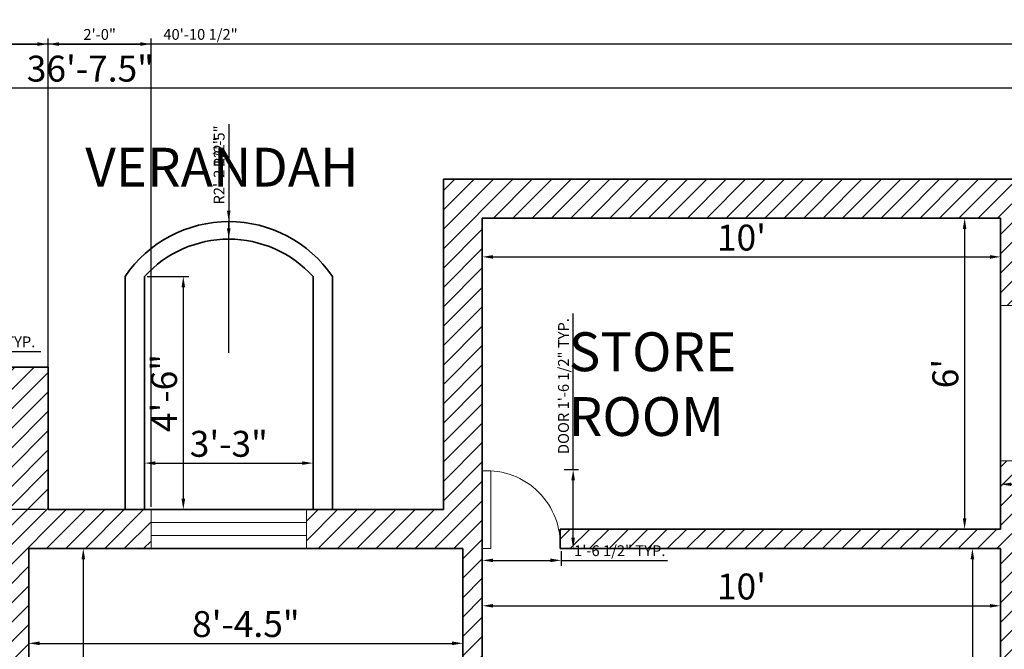
# Model space of a CAD drawing. Units: inches. Extents: x 4740 to 5323, y 7115 to 7713.
# Tile 5 of 6: x 4980 to 5208, y 7567 to 7713. Entities that reach past the tile are written whole.
import ezdxf

# ---------------------------------------------------------------- set-up
doc = ezdxf.new("R2010")
doc.units = ezdxf.units.IN
for name, color, linetype, lineweight in [('A-ANNO-DIMS', 2, 'Continuous', 18), ('A-AREA-IDEN', 7, 'Continuous', 25), ('A-DOOR', 4, 'Continuous', 18), ('A-GLAZ', 242, 'Continuous', 18), ('A-WALL', 7, 'Continuous', 35)]:
    doc.layers.add(name, color=color, linetype=linetype, lineweight=lineweight)
doc.layers.add('A-WALL-PATT', color=152, linetype='Continuous', lineweight=13, true_color=0x2776bb)
doc.styles.get("Standard").update_dxf_attribs({"font": 'arial.ttf'})
doc.dimstyles.new('ISO-25', dxfattribs={"dimtxt": 2.5, "dimasz": 2.5, "dimexe": 1.25, "dimexo": 0.625, "dimtad": 1, "dimlunit": 3, "dimtxsty": 'Standard', "dimcen": 2.5, "dimadec": 0, "dimazin": 0, "dimtfac": 1, "dimtmove": 0, "dimatfit": 3, "dimfxl": 1, "dimarcsym": 0})

# ---------------------------------------------------------------- blocks, each defined once
blk = doc.blocks.new('*D17')
at = {"layer": 'A-ANNO-DIMS', "color": 0, "lineweight": -2, "transparency": 16777216}
for p, q in [((5009.38, 7653.36), (5018.98, 7653.36)), ((5017.73, 7650.86), (5017.73, 7601.86)), ((5009.38, 7599.36), (5018.98, 7599.36))]:
    blk.add_line(p, q, dxfattribs=at)
at = {"layer": 'A-ANNO-DIMS', "color": 0, "transparency": 16777216}
for points in [[(5017.32, 7650.86), (5018.15, 7650.86), (5017.73, 7653.36)], [(5017.32, 7601.86), (5018.15, 7601.86), (5017.73, 7599.36)]]:
    blk.add_solid(points, dxfattribs=at)
at = {"layer": 'Defpoints', "color": 0, "transparency": 16777216}
for p in [(5008.76, 7653.36), (5008.76, 7599.36), (5017.73, 7599.36)]:
    blk.add_point(p, dxfattribs=at)
at = {"layer": 'A-ANNO-DIMS', "color": 0, "transparency": 16777216, "insert": (5014.05, 7626.36), "char_height": 6, "attachment_point": 5, "rotation": 90}
blk.add_mtext('4\'-6"', dxfattribs=at)
blk = doc.blocks.new('*D18')
at = {"layer": 'A-ANNO-DIMS', "color": 0, "lineweight": -2, "transparency": 16777216}
for p, q in [((5008.76, 7599.98), (5008.76, 7611.38)), ((5047.76, 7599.98), (5047.76, 7611.38)), ((5011.26, 7610.13), (5045.26, 7610.13))]:
    blk.add_line(p, q, dxfattribs=at)
at = {"layer": 'A-ANNO-DIMS', "color": 0, "transparency": 16777216}
for points in [[(5011.26, 7610.54), (5011.26, 7609.71), (5008.76, 7610.13)], [(5045.26, 7610.54), (5045.26, 7609.71), (5047.76, 7610.13)]]:
    blk.add_solid(points, dxfattribs=at)
at = {"layer": 'Defpoints', "color": 0, "transparency": 16777216}
for p in [(5047.76, 7610.13), (5008.76, 7599.36), (5047.76, 7599.36)]:
    blk.add_point(p, dxfattribs=at)
at = {"layer": 'A-ANNO-DIMS', "color": 0, "transparency": 16777216, "insert": (5028.26, 7613.82), "char_height": 6, "attachment_point": 5}
blk.add_mtext('3\'-3"', dxfattribs=at)
blk = doc.blocks.new('*D19')
at = {"layer": 'A-ANNO-DIMS', "color": 0, "lineweight": -2, "transparency": 16777216}
for p, q in [((5086.96, 7666.23), (5086.96, 7656.63)), ((5206.96, 7666.23), (5206.96, 7656.63)), ((5089.46, 7657.88), (5204.46, 7657.88))]:
    blk.add_line(p, q, dxfattribs=at)
at = {"layer": 'A-ANNO-DIMS', "color": 0, "transparency": 16777216}
for points in [[(5089.46, 7658.29), (5089.46, 7657.46), (5086.96, 7657.88)], [(5204.46, 7658.29), (5204.46, 7657.46), (5206.96, 7657.88)]]:
    blk.add_solid(points, dxfattribs=at)
at = {"layer": 'Defpoints', "color": 0, "transparency": 16777216}
for p in [(5086.96, 7666.86), (5206.96, 7666.86), (5206.96, 7657.88)]:
    blk.add_point(p, dxfattribs=at)
at = {"layer": 'A-ANNO-DIMS', "color": 0, "transparency": 16777216, "insert": (5146.96, 7661.57), "char_height": 6, "attachment_point": 5}
blk.add_mtext("10'", dxfattribs=at)
blk = doc.blocks.new('*D20')
at = {"layer": 'A-ANNO-DIMS', "color": 0, "lineweight": -2, "transparency": 16777216}
for p, q in [((5206.33, 7666.86), (5197.37, 7666.86)), ((5198.62, 7664.36), (5198.62, 7597.36)), ((5206.33, 7594.86), (5197.37, 7594.86))]:
    blk.add_line(p, q, dxfattribs=at)
at = {"layer": 'A-ANNO-DIMS', "color": 0, "transparency": 16777216}
for points in [[(5198.2, 7664.36), (5199.03, 7664.36), (5198.62, 7666.86)], [(5198.2, 7597.36), (5199.03, 7597.36), (5198.62, 7594.86)]]:
    blk.add_solid(points, dxfattribs=at)
at = {"layer": 'Defpoints', "color": 0, "transparency": 16777216}
for p in [(5206.96, 7666.86), (5198.62, 7594.86), (5206.96, 7594.86)]:
    blk.add_point(p, dxfattribs=at)
at = {"layer": 'A-ANNO-DIMS', "color": 0, "transparency": 16777216, "insert": (5194.93, 7630.86), "char_height": 6, "attachment_point": 5, "rotation": 90}
blk.add_mtext("6'", dxfattribs=at)
blk = doc.blocks.new('*D21')
at = {"layer": 'A-ANNO-DIMS', "color": 0, "lineweight": -2, "transparency": 16777216}
for p, q in [((5086.96, 7589.73), (5086.96, 7575.84)), ((5206.96, 7589.73), (5206.96, 7575.84)), ((5089.46, 7577.09), (5204.46, 7577.09))]:
    blk.add_line(p, q, dxfattribs=at)
at = {"layer": 'A-ANNO-DIMS', "color": 0, "transparency": 16777216}
for points in [[(5089.46, 7577.51), (5089.46, 7576.68), (5086.96, 7577.09)], [(5204.46, 7577.51), (5204.46, 7576.68), (5206.96, 7577.09)]]:
    blk.add_solid(points, dxfattribs=at)
at = {"layer": 'Defpoints', "color": 0, "transparency": 16777216}
for p in [(5086.96, 7590.36), (5206.96, 7590.36), (5206.96, 7577.09)]:
    blk.add_point(p, dxfattribs=at)
at = {"layer": 'A-ANNO-DIMS', "color": 0, "transparency": 16777216, "insert": (5146.96, 7580.78), "char_height": 6, "attachment_point": 5}
blk.add_mtext("10'", dxfattribs=at)
blk = doc.blocks.new('*D22')
at = {"layer": 'A-ANNO-DIMS', "color": 0, "lineweight": -2, "transparency": 16777216}
for p, q in [((5206.33, 7590.36), (5199.17, 7590.36)), ((5200.42, 7587.86), (5200.42, 7429.36)), ((5206.33, 7426.86), (5199.17, 7426.86))]:
    blk.add_line(p, q, dxfattribs=at)
at = {"layer": 'A-ANNO-DIMS', "color": 0, "transparency": 16777216}
for points in [[(5200, 7587.86), (5200.84, 7587.86), (5200.42, 7590.36)], [(5200, 7429.36), (5200.84, 7429.36), (5200.42, 7426.86)]]:
    blk.add_solid(points, dxfattribs=at)
at = {"layer": 'Defpoints', "color": 0, "transparency": 16777216}
for p in [(5206.96, 7590.36), (5200.42, 7426.86), (5206.96, 7426.86)]:
    blk.add_point(p, dxfattribs=at)
at = {"layer": 'A-ANNO-DIMS', "color": 0, "transparency": 16777216, "insert": (5196.73, 7508.61), "char_height": 6, "attachment_point": 5, "rotation": 90}
blk.add_mtext('13\'-7.5"', dxfattribs=at)
blk = doc.blocks.new('*D32')
at = {"layer": 'A-ANNO-DIMS', "color": 0, "lineweight": -2, "transparency": 16777216}
for p, q in [((4982.58, 7590.36), (4995.83, 7590.36)), ((4994.58, 7587.86), (4994.58, 7429.36)), ((4982.58, 7426.86), (4995.83, 7426.86))]:
    blk.add_line(p, q, dxfattribs=at)
at = {"layer": 'A-ANNO-DIMS', "color": 0, "transparency": 16777216}
for points in [[(4994.17, 7587.86), (4995, 7587.86), (4994.58, 7590.36)], [(4994.17, 7429.36), (4995, 7429.36), (4994.58, 7426.86)]]:
    blk.add_solid(points, dxfattribs=at)
at = {"layer": 'Defpoints', "color": 0, "transparency": 16777216}
for p in [(4981.96, 7590.36), (4981.96, 7426.86), (4994.58, 7426.86)]:
    blk.add_point(p, dxfattribs=at)
at = {"layer": 'A-ANNO-DIMS', "color": 0, "transparency": 16777216, "insert": (4990.89, 7508.61), "char_height": 6, "attachment_point": 5, "rotation": 90}
blk.add_mtext('13\'-7.5"', dxfattribs=at)
blk = doc.blocks.new('*D33')
at = {"layer": 'A-ANNO-DIMS', "color": 0, "lineweight": -2, "transparency": 16777216}
for p, q in [((4981.96, 7589.73), (4981.96, 7567.15)), ((5082.46, 7589.73), (5082.46, 7567.15)), ((4984.46, 7568.4), (5079.96, 7568.4))]:
    blk.add_line(p, q, dxfattribs=at)
at = {"layer": 'A-ANNO-DIMS', "color": 0, "transparency": 16777216}
for points in [[(4984.46, 7568.82), (4984.46, 7567.98), (4981.96, 7568.4)], [(5079.96, 7568.82), (5079.96, 7567.98), (5082.46, 7568.4)]]:
    blk.add_solid(points, dxfattribs=at)
at = {"layer": 'Defpoints', "color": 0, "transparency": 16777216}
for p in [(4981.96, 7590.36), (5082.46, 7590.36), (5082.46, 7568.4)]:
    blk.add_point(p, dxfattribs=at)
at = {"layer": 'A-ANNO-DIMS', "color": 0, "transparency": 16777216, "insert": (5032.21, 7572.09), "char_height": 6, "attachment_point": 5}
blk.add_mtext('8\'-4.5"', dxfattribs=at)
blk = doc.blocks.new('*D35')
at = {"layer": 'A-ANNO-DIMS', "color": 0, "lineweight": -2, "transparency": 16777216}
for p, q in [((4776.46, 7632.98), (4776.46, 7698.25)), ((5215.96, 7629.25), (5215.96, 7698.25)), ((4778.96, 7697), (5213.46, 7697))]:
    blk.add_line(p, q, dxfattribs=at)
at = {"layer": 'A-ANNO-DIMS', "color": 0, "transparency": 16777216}
for points in [[(4778.96, 7697.42), (4778.96, 7696.58), (4776.46, 7697)], [(5213.46, 7697.42), (5213.46, 7696.58), (5215.96, 7697)]]:
    blk.add_solid(points, dxfattribs=at)
at = {"layer": 'Defpoints', "color": 0, "transparency": 16777216}
for p in [(5215.96, 7697), (4776.46, 7632.36), (5215.96, 7628.62)]:
    blk.add_point(p, dxfattribs=at)
at = {"layer": 'A-ANNO-DIMS', "color": 0, "transparency": 16777216, "insert": (4996.21, 7700.69), "char_height": 6, "attachment_point": 5}
blk.add_mtext('36\'-7.5"', dxfattribs=at)
blk = doc.blocks.new('*D36')
at = {"layer": 'A-ANNO-DIMS', "color": 0, "lineweight": -2, "transparency": 16777216}
for p, q in [((5078.58, 7675.86), (5323.05, 7675.86)), ((5321.8, 7673.36), (5321.8, 7150.66)), ((5077.56, 7148.16), (5323.05, 7148.16))]:
    blk.add_line(p, q, dxfattribs=at)
at = {"layer": 'A-ANNO-DIMS', "color": 0, "transparency": 16777216}
for points in [[(5321.38, 7673.36), (5322.22, 7673.36), (5321.8, 7675.86)], [(5321.38, 7150.66), (5322.22, 7150.66), (5321.8, 7148.16)]]:
    blk.add_solid(points, dxfattribs=at)
at = {"layer": 'Defpoints', "color": 0, "transparency": 16777216}
for p in [(5077.96, 7675.86), (5076.93, 7148.16), (5321.8, 7148.16)]:
    blk.add_point(p, dxfattribs=at)
at = {"layer": 'A-ANNO-DIMS', "color": 0, "transparency": 16777216, "insert": (5318.11, 7412.01), "char_height": 6, "attachment_point": 5, "rotation": 90}
blk.add_mtext('43\'-11.7"', dxfattribs=at)
blk = doc.blocks.new('WIN-36IN')
for p, q in [((0, 36), (9, 36)), ((0, 36), (0, 0)), ((3, 36), (3, 0)), ((6, 36), (6, 0)), ((9, 0), (9, 36)), ((0, 0), (9, 0))]:
    blk.add_line(p, q)
blk = doc.blocks.new('DOOR-SWING-18IN')
for p, q in [((0, 0), (0, 18)), ((0, 18), (2, 18)), ((2, 18), (2, 0)), ((2, 0), (0, 0))]:
    blk.add_line(p, q)
blk.add_arc((1, 1), 17.03, 356.6335, 93.3665)
blk = doc.blocks.new('*D44')
at = {"layer": 'A-ANNO-DIMS', "color": 0, "lineweight": -2, "transparency": 16777216}
for p, q in [((4925.34, 7632.98), (4925.34, 7637.21)), ((4949.34, 7632.98), (4949.34, 7637.21)), ((4927.84, 7635.96), (4946.84, 7635.96)), ((4949.34, 7635.96), (4984.73, 7635.96))]:
    blk.add_line(p, q, dxfattribs=at)
at = {"layer": 'A-ANNO-DIMS', "color": 0, "transparency": 16777216}
for points in [[(4927.84, 7636.37), (4927.84, 7635.54), (4925.34, 7635.96)], [(4946.84, 7636.37), (4946.84, 7635.54), (4949.34, 7635.96)]]:
    blk.add_solid(points, dxfattribs=at)
at = {"layer": 'Defpoints', "color": 0, "transparency": 16777216}
for p in [(4949.34, 7635.96), (4925.34, 7632.36), (4949.34, 7632.36)]:
    blk.add_point(p, dxfattribs=at)
at = {"layer": 'A-ANNO-DIMS', "color": 0, "transparency": 16777216, "insert": (4968.29, 7637.88), "char_height": 2.5, "attachment_point": 5}
blk.add_mtext('WINDOW 2\'-0" TYP.', dxfattribs=at)
blk = doc.blocks.new('*D47')
at = {"layer": 'A-ANNO-DIMS', "color": 0, "lineweight": -2, "transparency": 16777216}
for p, q in [((5206.96, 7610), (5206.96, 7603.97)), ((5215.96, 7610), (5215.96, 7603.97)), ((5209.46, 7605.22), (5213.46, 7605.22)), ((5215.96, 7605.22), (5234.95, 7605.22))]:
    blk.add_line(p, q, dxfattribs=at)
at = {"layer": 'A-ANNO-DIMS', "color": 0, "transparency": 16777216}
for points in [[(5209.46, 7605.64), (5209.46, 7604.81), (5206.96, 7605.22)], [(5213.46, 7605.64), (5213.46, 7604.81), (5215.96, 7605.22)]]:
    blk.add_solid(points, dxfattribs=at)
at = {"layer": 'Defpoints', "color": 0, "transparency": 16777216}
for p in [(5206.96, 7610.62), (5215.96, 7610.62), (5215.96, 7605.22)]:
    blk.add_point(p, dxfattribs=at)
at = {"layer": 'A-ANNO-DIMS', "color": 0, "transparency": 16777216, "insert": (5226.7, 7607.13), "char_height": 2.5, "attachment_point": 5}
blk.add_mtext('0\'-9" TYP.', dxfattribs=at)
blk = doc.blocks.new('*D56')
at = {"layer": 'A-ANNO-DIMS', "color": 0, "lineweight": -2, "transparency": 16777216}
for p, q in [((5107.99, 7608.64), (5107.99, 7644.78)), ((5105.87, 7608.64), (5109.24, 7608.64)), ((5107.99, 7592.86), (5107.99, 7606.14)), ((5105.87, 7590.36), (5109.24, 7590.36))]:
    blk.add_line(p, q, dxfattribs=at)
at = {"layer": 'A-ANNO-DIMS', "color": 0, "transparency": 16777216}
for points in [[(5107.57, 7606.14), (5108.4, 7606.14), (5107.99, 7608.64)], [(5107.57, 7592.86), (5108.4, 7592.86), (5107.99, 7590.36)]]:
    blk.add_solid(points, dxfattribs=at)
at = {"layer": 'Defpoints', "color": 0, "transparency": 16777216}
for p in [(5105.24, 7608.64), (5107.99, 7608.64), (5105.24, 7590.36)]:
    blk.add_point(p, dxfattribs=at)
at = {"layer": 'A-ANNO-DIMS', "color": 0, "transparency": 16777216, "insert": (5106.07, 7627.96), "char_height": 2.5, "attachment_point": 5, "rotation": 90}
blk.add_mtext('DOOR 1\'-6 1/2" TYP.', dxfattribs=at)
blk = doc.blocks.new('*D57')
at = {"layer": 'A-ANNO-DIMS', "color": 0, "lineweight": -2, "transparency": 16777216}
for p, q in [((5086.96, 7589.73), (5086.96, 7586.36)), ((5105.24, 7589.73), (5105.24, 7586.36)), ((5089.46, 7587.61), (5102.74, 7587.61)), ((5105.24, 7587.61), (5129.82, 7587.61))]:
    blk.add_line(p, q, dxfattribs=at)
at = {"layer": 'A-ANNO-DIMS', "color": 0, "transparency": 16777216}
for points in [[(5089.46, 7588.03), (5089.46, 7587.2), (5086.96, 7587.61)], [(5102.74, 7588.03), (5102.74, 7587.2), (5105.24, 7587.61)]]:
    blk.add_solid(points, dxfattribs=at)
at = {"layer": 'Defpoints', "color": 0, "transparency": 16777216}
for p in [(5086.96, 7590.36), (5105.24, 7590.36), (5105.24, 7587.61)]:
    blk.add_point(p, dxfattribs=at)
at = {"layer": 'A-ANNO-DIMS', "color": 0, "transparency": 16777216, "insert": (5118.78, 7589.53), "char_height": 2.5, "attachment_point": 5}
blk.add_mtext('1\'-6 1/2" TYP.', dxfattribs=at)
blk = doc.blocks.new('*D74')
at = {"layer": 'A-ANNO-DIMS', "color": 0, "lineweight": -2, "transparency": 16777216}
for p, q in [((4949.34, 7632.98), (4949.34, 7708.41)), ((4951.84, 7707.16), (4983.96, 7707.16)), ((4986.46, 7632.98), (4986.46, 7708.41))]:
    blk.add_line(p, q, dxfattribs=at)
at = {"layer": 'A-ANNO-DIMS', "color": 0, "transparency": 16777216}
for points in [[(4951.84, 7707.57), (4951.84, 7706.74), (4949.34, 7707.16)], [(4983.96, 7707.57), (4983.96, 7706.74), (4986.46, 7707.16)]]:
    blk.add_solid(points, dxfattribs=at)
at = {"layer": 'Defpoints', "color": 0, "transparency": 16777216}
for p in [(4986.46, 7707.16), (4949.34, 7632.36), (4986.46, 7632.36)]:
    blk.add_point(p, dxfattribs=at)
at = {"layer": 'A-ANNO-DIMS', "color": 0, "transparency": 16777216, "insert": (4967.9, 7709.06), "char_height": 2.5, "attachment_point": 5}
blk.add_mtext('3\'-1"', dxfattribs=at)
blk = doc.blocks.new('*D80')
at = {"layer": 'A-ANNO-DIMS', "color": 0, "lineweight": -2, "transparency": 16777216}
for p, q in [((4986.46, 7599.98), (4986.46, 7708.41)), ((4988.96, 7707.16), (5007.76, 7707.16)), ((5010.26, 7599.98), (5010.26, 7708.41))]:
    blk.add_line(p, q, dxfattribs=at)
at = {"layer": 'A-ANNO-DIMS', "color": 0, "transparency": 16777216}
for points in [[(4988.96, 7707.57), (4988.96, 7706.74), (4986.46, 7707.16)], [(5007.76, 7707.57), (5007.76, 7706.74), (5010.26, 7707.16)]]:
    blk.add_solid(points, dxfattribs=at)
at = {"layer": 'Defpoints', "color": 0, "transparency": 16777216}
for p in [(5010.26, 7707.16), (4986.46, 7599.36), (5010.26, 7599.36)]:
    blk.add_point(p, dxfattribs=at)
at = {"layer": 'A-ANNO-DIMS', "color": 0, "transparency": 16777216, "insert": (4998.36, 7709.06), "char_height": 2.5, "attachment_point": 5}
blk.add_mtext('2\'-0"', dxfattribs=at)
blk = doc.blocks.new('*D81')
at = {"layer": 'A-ANNO-DIMS', "color": 0, "lineweight": -2, "transparency": 16777216}
for p, q in [((4776.46, 7632.98), (4776.46, 7708.41)), ((5264.46, 7707.16), (4778.96, 7707.16)), ((5266.96, 7422.98), (5266.96, 7708.41))]:
    blk.add_line(p, q, dxfattribs=at)
at = {"layer": 'A-ANNO-DIMS', "color": 0, "transparency": 16777216}
for points in [[(4778.96, 7707.57), (4778.96, 7706.74), (4776.46, 7707.16)], [(5264.46, 7707.57), (5264.46, 7706.74), (5266.96, 7707.16)]]:
    blk.add_solid(points, dxfattribs=at)
at = {"layer": 'Defpoints', "color": 0, "transparency": 16777216}
for p in [(4776.46, 7707.16), (4776.46, 7632.36), (5266.96, 7422.36)]:
    blk.add_point(p, dxfattribs=at)
at = {"layer": 'A-ANNO-DIMS', "color": 0, "transparency": 16777216, "insert": (5021.71, 7709.07), "char_height": 2.5, "attachment_point": 5}
blk.add_mtext('40\'-10 1/2"', dxfattribs=at)
blk = doc.blocks.new('*D82')
at = {"layer": 'A-ANNO-DIMS', "color": 0, "lineweight": -2, "transparency": 16777216}
for p, q in [((4985.83, 7632.36), (4743.91, 7632.36)), ((4745.16, 7629.86), (4745.16, 7601.86)), ((4985.83, 7599.36), (4743.91, 7599.36))]:
    blk.add_line(p, q, dxfattribs=at)
at = {"layer": 'A-ANNO-DIMS', "color": 0, "transparency": 16777216}
for points in [[(4744.74, 7629.86), (4745.58, 7629.86), (4745.16, 7632.36)], [(4744.74, 7601.86), (4745.58, 7601.86), (4745.16, 7599.36)]]:
    blk.add_solid(points, dxfattribs=at)
at = {"layer": 'Defpoints', "color": 0, "transparency": 16777216}
for p in [(4986.46, 7632.36), (4745.16, 7599.36), (4986.46, 7599.36)]:
    blk.add_point(p, dxfattribs=at)
at = {"layer": 'A-ANNO-DIMS', "color": 0, "transparency": 16777216, "insert": (4743.26, 7615.86), "char_height": 2.5, "attachment_point": 5, "rotation": 90}
blk.add_mtext('2\'-9"', dxfattribs=at)
blk = doc.blocks.new('*D86')
at = {"layer": 'A-ANNO-DIMS', "color": 0, "lineweight": -2, "transparency": 16777216}
for p, q in [((5028.26, 7688.62), (5028.26, 7668.56)), ((5028.26, 7637.03), (5028.26, 7666.06))]:
    blk.add_line(p, q, dxfattribs=at)
at = {"layer": 'A-ANNO-DIMS', "color": 0, "transparency": 16777216}
blk.add_solid([(5027.84, 7668.56), (5028.67, 7668.56), (5028.26, 7666.06)], dxfattribs=at)
at = {"layer": 'Defpoints', "color": 0, "transparency": 16777216}
for p in [(5028.26, 7666.06), (5028.26, 7637.03)]:
    blk.add_point(p, dxfattribs=at)
at = {"layer": 'A-ANNO-DIMS', "color": 0, "transparency": 16777216, "insert": (5026.36, 7683.47), "char_height": 2.5, "attachment_point": 5, "rotation": 89.9991}
blk.add_mtext('R2\'-5"', dxfattribs=at)
blk = doc.blocks.new('*D87')
at = {"layer": 'A-ANNO-DIMS', "color": 0, "lineweight": -2, "transparency": 16777216}
for p, q in [((5028.26, 7685.85), (5028.26, 7664.49)), ((5028.26, 7635.64), (5028.26, 7661.99))]:
    blk.add_line(p, q, dxfattribs=at)
at = {"layer": 'A-ANNO-DIMS', "color": 0, "transparency": 16777216}
blk.add_solid([(5027.84, 7664.49), (5028.67, 7664.49), (5028.26, 7661.99)], dxfattribs=at)
at = {"layer": 'Defpoints', "color": 0, "transparency": 16777216}
for p in [(5028.26, 7661.99), (5028.26, 7635.64)]:
    blk.add_point(p, dxfattribs=at)
at = {"layer": 'A-ANNO-DIMS', "color": 0, "transparency": 16777216, "insert": (5026.34, 7677.79), "char_height": 2.5, "attachment_point": 5, "rotation": 89.999}
blk.add_mtext('R2\'-2 1/2"', dxfattribs=at)

msp = doc.modelspace()

# ---------------------------------------------------------------- hatches: boundary and pattern name
at = {"layer": 'A-WALL-PATT'}
h = msp.add_hatch(dxfattribs=at)
h.set_pattern_fill('ANSI31', color=256)
h.paths.add_polyline_path([(4925.343, 7632.357), (4776.459, 7632.357), (4776.459, 7486.448), (4785.459, 7486.448), (4785.459, 7522.857), (4959.459, 7522.857), (4959.459, 7527.357), (4785.459, 7527.357), (4785.459, 7623.357), (4833.459, 7623.357), (4925.343, 7623.357)])
h.paths.add_polyline_path([(5010.258, 7599.357), (5004.258, 7599.357), (4986.459, 7599.357), (4986.459, 7623.357), (4986.459, 7632.357), (4977.459, 7632.357), (4949.343, 7632.357), (4949.343, 7623.357), (4977.459, 7623.357), (4977.459, 7599.357), (4977.459, 7594.857), (4977.459, 7590.357), (4977.459, 7524.857, -0.0293864), (4977.459, 7522.857), (4977.459, 7426.857), (4977.459, 7422.357), (4977.459, 7419.778), (4981.959, 7419.778), (4981.959, 7422.357), (5041.959, 7422.357), (5041.959, 7479.357), (5037.459, 7479.357), (5037.459, 7426.857), (4981.959, 7426.857), (4981.959, 7590.357), (5010.258, 7590.357)])
h.paths.add_polyline_path([(5086.959, 7666.857), (5206.959, 7666.857), (5206.959, 7646.624), (5215.959, 7646.624), (5215.959, 7675.857), (5077.959, 7675.857), (5077.959, 7599.357), (5046.258, 7599.357), (5046.258, 7590.357), (5082.459, 7590.357), (5082.459, 7474.857, -0.0106371), (5084.459, 7474.857), (5086.959, 7474.857)])
h.paths.add_polyline_path([(5215.959, 7610.624), (5206.959, 7610.624), (5206.959, 7594.857), (5104.959, 7594.857), (5104.959, 7592.357, -0.0293864), (5104.959, 7590.357), (5206.959, 7590.357), (5206.959, 7426.857), (5104.959, 7426.857), (5082.459, 7426.857), (5082.459, 7422.357), (5104.959, 7422.357), (5215.959, 7422.357), (5215.959, 7464.357), (5215.959, 7506.357)])
h.paths.add_polyline_path([(4881.459, 7375.857), (4977.459, 7375.857), (4977.459, 7296.657), (4981.959, 7296.657), (4981.959, 7384.857), (4951.959, 7384.857), (4785.459, 7384.857), (4785.459, 7438.448), (4776.459, 7438.448), (4776.459, 7375.857), (4872.459, 7375.857), (4872.459, 7337.044), (4881.459, 7337.044)])
h.paths.add_polyline_path([(4881.459, 7313.044), (4872.459, 7313.044), (4872.459, 7148.157), (4916.568, 7148.157), (4916.568, 7157.157), (4881.459, 7157.157), (4881.459, 7269.357), (4981.959, 7269.357), (4981.959, 7273.857), (4963.959, 7273.857), (4881.459, 7273.857)])
h.paths.add_polyline_path([(5029.959, 7296.657), (5116.509, 7296.657), (5116.509, 7299.157, -0.0121933), (5116.509, 7301.157), (5025.459, 7301.157), (5025.459, 7157.157), (4964.568, 7157.157), (4964.568, 7148.157), (5076.933, 7148.157), (5076.933, 7157.157), (5029.959, 7157.157)])
h.paths.add_polyline_path([(5182.959, 7203.442), (5173.959, 7203.442), (5173.959, 7157.157), (5124.933, 7157.157), (5124.933, 7148.157), (5182.959, 7148.157)])
h.paths.add_polyline_path([(5266.959, 7353.764), (5257.959, 7353.764), (5257.959, 7301.157), (5182.959, 7301.157), (5158.509, 7301.157), (5158.509, 7296.657), (5173.959, 7296.657), (5173.959, 7263.442), (5182.959, 7263.442), (5182.959, 7292.157), (5266.959, 7292.157)])
h.paths.add_polyline_path([(5266.959, 7422.357), (5257.959, 7422.357), (5257.959, 7377.764), (5266.959, 7377.764)])

# ---------------------------------------------------------------- linework, layer by layer
at = {"layer": 'A-WALL'}
for p, q in [((5077.959, 7675.857), (5077.959, 7599.357)), ((5077.959, 7675.857), (5215.959, 7675.857)), ((5086.959, 7666.857), (5086.959, 7474.857)), ((5086.959, 7666.857), (5206.959, 7666.857)), ((5206.959, 7666.857), (5206.959, 7594.857)), ((5004.258, 7599.357), (5004.258, 7653.357)), ((5004.258, 7653.357), (5004.258, 7653.357)), ((5008.758, 7599.357), (5008.758, 7653.357)), ((5047.758, 7599.357), (5047.758, 7653.357)), ((5052.258, 7599.357), (5052.258, 7653.357)), ((4977.459, 7632.357), (4986.459, 7632.357)), ((4986.459, 7632.357), (4986.459, 7623.357)), ((4986.459, 7599.357), (4986.459, 7623.357)), ((4986.459, 7599.357), (5077.959, 7599.357)), ((5010.258, 7599.357), (5004.258, 7599.357)), ((5010.258, 7599.357), (5004.258, 7599.357)), ((5046.258, 7599.357), (5052.258, 7599.357)), ((5104.959, 7594.857), (5206.959, 7594.857)), ((5104.959, 7594.857), (5104.959, 7590.357)), ((4981.959, 7590.357), (4981.959, 7426.857)), ((4981.959, 7590.357), (5082.459, 7590.357)), ((5082.459, 7590.357), (5082.459, 7474.857)), ((5104.959, 7590.357), (5206.959, 7590.357)), ((5206.959, 7590.357), (5206.959, 7426.857))]:
    msp.add_line(p, q, dxfattribs=at)
for centre, radius, start, end in [((5028.258, 7637.027), 29.029, 34.23166, 145.76834), ((5028.258, 7635.643), 26.345, 42.25276, 137.74724)]:
    msp.add_arc(centre, radius, start, end, dxfattribs=at)

# ---------------------------------------------------------------- block references
at = {"layer": 'A-DOOR'}
msp.add_blockref('DOOR-SWING-18IN', (5086.959, 7590.357), dxfattribs=at)
at = {"layer": 'A-GLAZ'}
msp.add_blockref('WIN-36IN', (5206.959, 7610.624), dxfattribs=at)
at = {"layer": 'A-GLAZ', "rotation": 89.99999999999181}
msp.add_blockref('WIN-36IN', (5046.258, 7590.357), dxfattribs=at)

# ---------------------------------------------------------------- texts
at = {"layer": 'A-AREA-IDEN', "char_height": 9, "attachment_point": 1}
for s, width, heights, insert in [('{ VERANDAH}', 75.84022, [0], (4992.296, 7683.153)), ('{ STORE        \\P ROOM}', 86.13245, [54.212], (5104.211, 7640.414))]:
    msp.add_mtext_dynamic_manual_height_columns(s, width=width, gutter_width=12.5, heights=heights, dxfattribs=dict(at, insert=insert))

# ---------------------------------------------------------------- dimensions: what is measured, and where the dimension line sits
at = {"layer": 'A-ANNO-DIMS'}
for base, p1, p2, override, picture, middle in [((4776.459, 7707.157), (5266.959, 7422.357), (4776.459, 7632.357), {"dimdec": 1, "dimlfac": 1, "dimrnd": 0, "dimzin": 1, "dimdsep": 46, "dimlunit": 4, "dimfrac": 2}, '*D81', (5021.709, 7709.074)), ((4986.459, 7707.157), (4949.343, 7632.357), (4986.459, 7632.357), {"dimdec": 1, "dimlfac": 1, "dimrnd": 0, "dimzin": 1, "dimdsep": 46, "dimlunit": 4, "dimfrac": 2}, '*D74', (4967.901, 7709.059)), ((5010.258, 7707.157), (4986.459, 7599.357), (5010.258, 7599.357), {"dimdec": 1, "dimlfac": 1, "dimrnd": 0, "dimzin": 1, "dimdsep": 46, "dimlunit": 4, "dimfrac": 2}, '*D80', (4998.358, 7709.058)), ((5215.959, 7697.001), (4776.459, 7632.357), (5215.959, 7628.624), {"dimtxt": 6, "dimclrd": 0, "dimclre": 0, "dimclrt": 0}, '*D35', (4996.209, 7700.692)), ((5206.959, 7657.878), (5086.959, 7666.857), (5206.959, 7666.857), {"dimtxt": 6, "dimclrd": 0, "dimclre": 0, "dimclrt": 0}, '*D19', (5146.959, 7661.566)), ((5047.758, 7610.125), (5008.758, 7599.357), (5047.758, 7599.357), {"dimtxt": 6, "dimclrd": 0, "dimclre": 0, "dimclrt": 0}, '*D18', (5028.258, 7613.816)), ((5082.459, 7568.4), (4981.959, 7590.357), (5082.459, 7590.357), {"dimtxt": 6, "dimclrd": 0, "dimclre": 0, "dimclrt": 0}, '*D33', (5032.209, 7572.089)), ((5206.959, 7577.093), (5086.959, 7590.357), (5206.959, 7590.357), {"dimtxt": 6, "dimclrd": 0, "dimclre": 0, "dimclrt": 0}, '*D21', (5146.959, 7580.782))]:
    dim = msp.add_linear_dim(base=base, p1=p1, p2=p2, dimstyle='ISO-25', override=override, dxfattribs=at)
    dim.commit()
    dim.dimension.update_dxf_attribs({"geometry": picture, "text_midpoint": middle})
for center, mpoint, picture, middle in [((5028.258, 7637.027), (5028.258, 7666.056), '*D86', (5028.258, 7683.473)), ((5028.258, 7635.643), (5028.258, 7661.987), '*D87', (5028.258, 7677.794))]:
    dim = msp.add_radius_dim(center=center, mpoint=mpoint, dimstyle='ISO-25', override={"dimdec": 1, "dimlfac": 1, "dimrnd": 0, "dimzin": 1, "dimdsep": 46, "dimlunit": 4, "dimfrac": 2}, dxfattribs=at)
    dim.commit()
    dim.dimension.update_dxf_attribs({"geometry": picture, "text_midpoint": middle, "dimtype": 164})
for base, p1, p2, override, picture, middle in [((5321.801, 7148.157), (5077.959, 7675.857), (5076.933, 7148.157), {"dimtxt": 6, "dimclrd": 0, "dimclre": 0, "dimclrt": 0}, '*D36', (5318.111, 7412.007)), ((5198.616, 7594.857), (5206.959, 7666.857), (5206.959, 7594.857), {"dimtxt": 6, "dimclrd": 0, "dimclre": 0, "dimclrt": 0}, '*D20', (5194.927, 7630.857)), ((4745.159, 7599.357), (4986.459, 7632.357), (4986.459, 7599.357), {"dimdec": 1, "dimlfac": 1, "dimrnd": 0, "dimzin": 1, "dimdsep": 46, "dimlunit": 4, "dimfrac": 2}, '*D82', (4743.258, 7615.857)), ((4994.583, 7426.857), (4981.959, 7590.357), (4981.959, 7426.857), {"dimtxt": 6, "dimclrd": 0, "dimclre": 0, "dimclrt": 0}, '*D32', (4990.893, 7508.607))]:
    dim = msp.add_linear_dim(base=base, p1=p1, p2=p2, angle=90, dimstyle='ISO-25', override=override, dxfattribs=at)
    dim.commit()
    dim.dimension.update_dxf_attribs({"geometry": picture, "text_midpoint": middle})
for base, p1, p2, picture, middle in [((5017.735, 7599.357), (5008.758, 7653.357), (5008.758, 7599.357), '*D17', (5017.735, 7626.357)), ((5200.419, 7426.857), (5206.959, 7590.357), (5206.959, 7426.857), '*D22', (5200.419, 7508.607))]:
    dim = msp.add_linear_dim(base=base, p1=p1, p2=p2, angle=90, dimstyle='ISO-25', override={"dimtxt": 6, "dimclrd": 0, "dimclre": 0, "dimclrt": 0}, dxfattribs=at)
    dim.commit()
    dim.dimension.update_dxf_attribs({"geometry": picture, "text_midpoint": middle, "dimtype": 160})
for base, p1, p2, angle, text, picture, middle in [((4949.343, 7635.957), (4925.343, 7632.357), (4949.343, 7632.357), 0, 'WINDOW <> TYP.', '*D44', (4968.286, 7637.875)), ((5107.988, 7608.642), (5105.245, 7590.357), (5105.245, 7608.642), 90, 'DOOR <> TYP.', '*D56', (5106.069, 7627.961))]:
    dim = msp.add_linear_dim(base=base, p1=p1, p2=p2, angle=angle, text=text, dimstyle='ISO-25', override={"dimdec": 1, "dimlfac": 1, "dimrnd": 0, "dimzin": 1, "dimdsep": 46, "dimlunit": 4, "dimfrac": 2}, dxfattribs=at)
    dim.commit()
    dim.dimension.update_dxf_attribs({"geometry": picture, "text_midpoint": middle})
for base, p1, p2, picture, middle in [((5215.959, 7605.224), (5206.959, 7610.624), (5215.959, 7610.624), '*D47', (5226.704, 7607.125)), ((5105.245, 7587.614), (5086.959, 7590.357), (5105.245, 7590.357), '*D57', (5118.784, 7589.532))]:
    dim = msp.add_linear_dim(base=base, p1=p1, p2=p2, text='<> TYP.', dimstyle='ISO-25', override={"dimdec": 1, "dimlfac": 1, "dimrnd": 0, "dimzin": 1, "dimdsep": 46, "dimlunit": 4, "dimfrac": 2}, dxfattribs=at)
    dim.commit()
    dim.dimension.update_dxf_attribs({"geometry": picture, "text_midpoint": middle})

doc.saveas('drawing.dxf')
